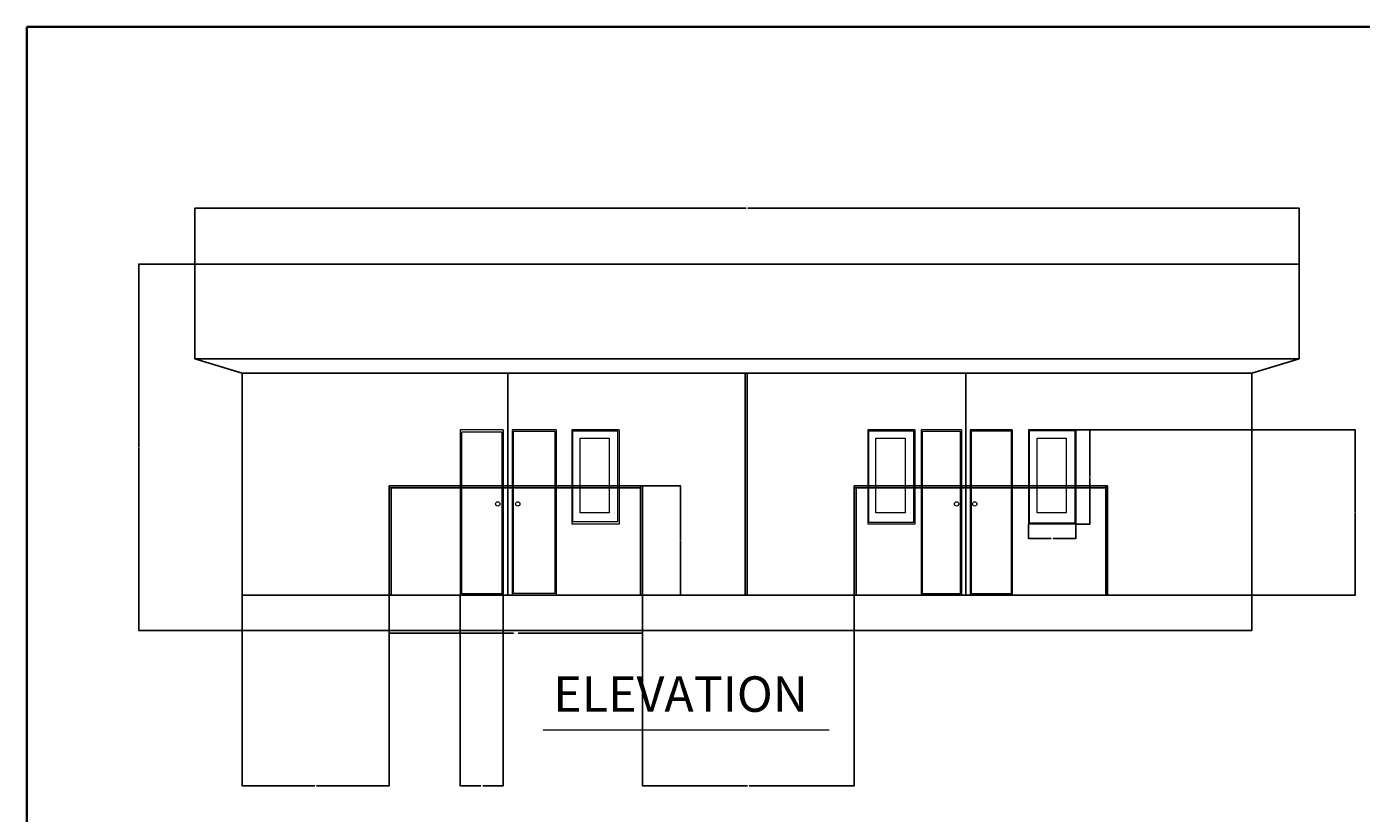
# Model space of a CAD drawing. Units: inches. Extents: x 2055 to 3558, y 1520 to 2888.
# Tile 4 of 8: x 2055 to 2732, y 2489 to 2888. Entities that reach past the tile are written whole.
import ezdxf

# ---------------------------------------------------------------- set-up
doc = ezdxf.new("R2010")
doc.units = ezdxf.units.IN
for name, color, linetype, lineweight in [('A-ANNO-DIMS', 2, 'Continuous', 18), ('A-ANNO-TEXT', 7, 'Continuous', 18), ('A-ANNO-TTLB', 7, 'Continuous', 35), ('A-ELEV', 7, 'Continuous', 25), ('A-ELEV-DOOR', 3, 'Continuous', 18), ('A-ELEV-GLAZ', 4, 'Continuous', 18)]:
    doc.layers.add(name, color=color, linetype=linetype, lineweight=lineweight)
doc.styles.get("Standard").update_dxf_attribs({"font": 'arial.ttf'})
doc.dimstyles.get("Standard").update_dxf_attribs({"dimtxt": 0.18, "dimasz": 0.18, "dimexe": 0.18, "dimexo": 0.0625, "dimgap": 0.09, "dimtad": 0, "dimtih": 1, "dimtoh": 1, "dimdec": 4, "dimzin": 0, "dimdsep": 46, "dimtxsty": 'Standard', "dimcen": 0.09, "dimadec": 0, "dimazin": 0, "dimtfac": 1, "dimtdec": 4, "dimtofl": 0, "dimtmove": 0, "dimatfit": 3, "dimfxl": 1, "dimtolj": 1, "dimtzin": 0, "dimarcsym": 0})

# ---------------------------------------------------------------- blocks, each defined once
blk = doc.blocks.new('VERANDA-FRONT-ELEV')
for p, q in [((0, 0), (0, 55.52)), ((0, 55.52), (128.65, 55.52)), ((127.65, 54.52), (0, 54.52)), ((0, 54.52), (1, 54.52)), ((1, 54.52), (1, 0)), ((127.65, 0), (127.65, 55.52)), ((127.65, 55.52), (127.65, 54.52)), ((128.65, 0), (128.65, 55.52)), ((128.65, 0), (127.65, 0))]:
    blk.add_line(p, q)
blk = doc.blocks.new('WIN-FRAME-ELEV-24')
for p, q in [((0, 48), (0, 0)), ((24, 48), (0, 48)), ((24, 48), (24, 0)), ((24, 0), (0, 0))]:
    blk.add_line(p, q)
blk = doc.blocks.new('*D50')
at = {"layer": 'A-ANNO-DIMS', "color": 0, "lineweight": -2, "transparency": 16777216}
for p, q in [((2587.37, 2683.6), (2594.69, 2683.6)), ((2594.51, 2683.42), (2594.51, 2659.78)), ((2594.51, 2635.78), (2594.51, 2659.42)), ((2587.37, 2635.6), (2594.69, 2635.6))]:
    blk.add_line(p, q, dxfattribs=at)
at = {"layer": 'A-ANNO-DIMS', "color": 0, "transparency": 16777216}
for points in [[(2594.48, 2683.42), (2594.54, 2683.42), (2594.51, 2683.6)], [(2594.48, 2635.78), (2594.54, 2635.78), (2594.51, 2635.6)]]:
    blk.add_solid(points, dxfattribs=at)
at = {"layer": 'Defpoints', "color": 0, "transparency": 16777216}
for p in [(2587.31, 2683.6), (2594.51, 2683.6), (2587.31, 2635.6)]:
    blk.add_point(p, dxfattribs=at)
at = {"layer": 'A-ANNO-DIMS', "color": 0, "transparency": 16777216, "insert": (2594.51, 2659.6), "char_height": 0.18, "attachment_point": 5}
blk.add_mtext('\\A1;WINDOW 48 TYP.', dxfattribs=at)
blk = doc.blocks.new('*D51')
at = {"layer": 'A-ANNO-DIMS', "color": 0, "lineweight": -2, "transparency": 16777216}
for p, q in [((2563.31, 2635.54), (2563.31, 2628.22)), ((2587.31, 2635.54), (2587.31, 2628.22)), ((2563.49, 2628.4), (2574.78, 2628.4)), ((2587.13, 2628.4), (2575.84, 2628.4))]:
    blk.add_line(p, q, dxfattribs=at)
at = {"layer": 'A-ANNO-DIMS', "color": 0, "transparency": 16777216}
for points in [[(2563.49, 2628.43), (2563.49, 2628.37), (2563.31, 2628.4)], [(2587.13, 2628.43), (2587.13, 2628.37), (2587.31, 2628.4)]]:
    blk.add_solid(points, dxfattribs=at)
at = {"layer": 'Defpoints', "color": 0, "transparency": 16777216}
for p in [(2563.31, 2635.6), (2587.31, 2635.6), (2587.31, 2628.4)]:
    blk.add_point(p, dxfattribs=at)
at = {"layer": 'A-ANNO-DIMS', "color": 0, "transparency": 16777216, "insert": (2575.31, 2628.4), "char_height": 0.18, "attachment_point": 5}
blk.add_mtext('\\A1;24 TYP.', dxfattribs=at)
blk = doc.blocks.new('*D116')
at = {"layer": 'A-ANNO-DIMS', "color": 0, "lineweight": -2, "transparency": 16777216}
for p, q in [((2238.74, 2599.54), (2238.74, 2580.12)), ((2367.39, 2599.54), (2367.39, 2580.12)), ((2238.92, 2580.3), (2301.82, 2580.3)), ((2367.21, 2580.3), (2304.31, 2580.3))]:
    blk.add_line(p, q, dxfattribs=at)
at = {"layer": 'A-ANNO-DIMS', "color": 0, "transparency": 16777216}
for points in [[(2238.92, 2580.33), (2238.92, 2580.27), (2238.74, 2580.3)], [(2367.21, 2580.33), (2367.21, 2580.27), (2367.39, 2580.3)]]:
    blk.add_solid(points, dxfattribs=at)
at = {"layer": 'Defpoints', "color": 0, "transparency": 16777216}
for p in [(2238.74, 2599.6), (2367.39, 2599.6), (2367.39, 2580.3)]:
    blk.add_point(p, dxfattribs=at)
at = {"layer": 'A-ANNO-DIMS', "color": 0, "transparency": 16777216, "insert": (2303.07, 2580.3), "char_height": 0.18, "attachment_point": 5}
blk.add_mtext('\\A1;VERANDA 129 TYP.', dxfattribs=at)
blk = doc.blocks.new('*D117')
at = {"layer": 'A-ANNO-DIMS', "color": 0, "lineweight": -2, "transparency": 16777216}
for p, q in [((2367.45, 2655.12), (2386.87, 2655.12)), ((2386.69, 2654.94), (2386.69, 2627.54)), ((2386.69, 2599.78), (2386.69, 2627.18)), ((2367.45, 2599.6), (2386.87, 2599.6))]:
    blk.add_line(p, q, dxfattribs=at)
at = {"layer": 'A-ANNO-DIMS', "color": 0, "transparency": 16777216}
for points in [[(2386.66, 2654.94), (2386.72, 2654.94), (2386.69, 2655.12)], [(2386.66, 2599.78), (2386.72, 2599.78), (2386.69, 2599.6)]]:
    blk.add_solid(points, dxfattribs=at)
at = {"layer": 'Defpoints', "color": 0, "transparency": 16777216}
for p in [(2367.39, 2655.12), (2386.69, 2655.12), (2367.39, 2599.6)]:
    blk.add_point(p, dxfattribs=at)
at = {"layer": 'A-ANNO-DIMS', "color": 0, "transparency": 16777216, "insert": (2386.69, 2627.36), "char_height": 0.18, "attachment_point": 5}
blk.add_mtext('\\A1;56 TYP.', dxfattribs=at)
blk = doc.blocks.new('*D143')
at = {"layer": 'A-ANNO-DIMS', "color": 0, "lineweight": -2, "transparency": 16777216}
for p, q in [((2140.17, 2767.66), (2140.17, 2796.23)), ((2140.35, 2796.05), (2420.03, 2796.05)), ((2700.49, 2796.05), (2420.82, 2796.05)), ((2700.67, 2767.66), (2700.67, 2796.23))]:
    blk.add_line(p, q, dxfattribs=at)
at = {"layer": 'A-ANNO-DIMS', "color": 0, "transparency": 16777216}
for points in [[(2140.35, 2796.08), (2140.35, 2796.02), (2140.17, 2796.05)], [(2700.49, 2796.08), (2700.49, 2796.02), (2700.67, 2796.05)]]:
    blk.add_solid(points, dxfattribs=at)
at = {"layer": 'Defpoints', "color": 0, "transparency": 16777216}
for p in [(2700.67, 2796.05), (2140.17, 2767.6), (2700.67, 2767.6)]:
    blk.add_point(p, dxfattribs=at)
at = {"layer": 'A-ANNO-DIMS', "color": 0, "transparency": 16777216, "insert": (2420.42, 2796.05), "char_height": 0.18, "attachment_point": 5}
blk.add_mtext('\\A1;560.5', dxfattribs=at)
blk = doc.blocks.new('*D144')
at = {"layer": 'A-ANNO-DIMS', "color": 0, "lineweight": -2, "transparency": 16777216}
for p, q in [((2140.11, 2767.6), (2111.54, 2767.6)), ((2111.72, 2767.42), (2111.72, 2674.78)), ((2111.72, 2581.78), (2111.72, 2674.42)), ((2164.11, 2581.6), (2111.54, 2581.6))]:
    blk.add_line(p, q, dxfattribs=at)
at = {"layer": 'A-ANNO-DIMS', "color": 0, "transparency": 16777216}
for points in [[(2111.69, 2767.42), (2111.75, 2767.42), (2111.72, 2767.6)], [(2111.69, 2581.78), (2111.75, 2581.78), (2111.72, 2581.6)]]:
    blk.add_solid(points, dxfattribs=at)
at = {"layer": 'Defpoints', "color": 0, "transparency": 16777216}
for p in [(2111.72, 2767.6), (2140.17, 2767.6), (2164.17, 2581.6)]:
    blk.add_point(p, dxfattribs=at)
at = {"layer": 'A-ANNO-DIMS', "color": 0, "transparency": 16777216, "insert": (2111.72, 2674.6), "char_height": 0.18, "attachment_point": 5}
blk.add_mtext('\\A1;186', dxfattribs=at)
blk = doc.blocks.new('*D145')
at = {"layer": 'A-ANNO-DIMS', "color": 0, "lineweight": -2, "transparency": 16777216}
for p, q in [((2164.17, 2599.54), (2164.17, 2502.58)), ((2238.74, 2599.54), (2238.74, 2502.58)), ((2164.35, 2502.76), (2201.07, 2502.76)), ((2238.56, 2502.76), (2201.85, 2502.76))]:
    blk.add_line(p, q, dxfattribs=at)
at = {"layer": 'A-ANNO-DIMS', "color": 0, "transparency": 16777216}
for points in [[(2164.35, 2502.79), (2164.35, 2502.73), (2164.17, 2502.76)], [(2238.56, 2502.79), (2238.56, 2502.73), (2238.74, 2502.76)]]:
    blk.add_solid(points, dxfattribs=at)
at = {"layer": 'Defpoints', "color": 0, "transparency": 16777216}
for p in [(2164.17, 2599.6), (2238.74, 2599.6), (2238.74, 2502.76)]:
    blk.add_point(p, dxfattribs=at)
at = {"layer": 'A-ANNO-DIMS', "color": 0, "transparency": 16777216, "insert": (2201.46, 2502.76), "char_height": 0.18, "attachment_point": 5}
blk.add_mtext('\\A1;74.57', dxfattribs=at)
blk = doc.blocks.new('*D146')
at = {"layer": 'A-ANNO-DIMS', "color": 0, "lineweight": -2, "transparency": 16777216}
for p, q in [((2367.39, 2599.54), (2367.39, 2502.58)), ((2474.84, 2599.54), (2474.84, 2502.58)), ((2367.57, 2502.76), (2420.66, 2502.76)), ((2474.66, 2502.76), (2421.57, 2502.76))]:
    blk.add_line(p, q, dxfattribs=at)
at = {"layer": 'A-ANNO-DIMS', "color": 0, "transparency": 16777216}
for points in [[(2367.57, 2502.79), (2367.57, 2502.73), (2367.39, 2502.76)], [(2474.66, 2502.79), (2474.66, 2502.73), (2474.84, 2502.76)]]:
    blk.add_solid(points, dxfattribs=at)
at = {"layer": 'Defpoints', "color": 0, "transparency": 16777216}
for p in [(2367.39, 2599.6), (2474.84, 2599.6), (2474.84, 2502.76)]:
    blk.add_point(p, dxfattribs=at)
at = {"layer": 'A-ANNO-DIMS', "color": 0, "transparency": 16777216, "insert": (2421.12, 2502.76), "char_height": 0.18, "attachment_point": 5}
blk.add_mtext('\\A1;107.45', dxfattribs=at)
blk = doc.blocks.new('*D147')
at = {"layer": 'A-ANNO-DIMS', "color": 0, "lineweight": -2, "transparency": 16777216}
for p, q in [((2274.85, 2599.54), (2274.85, 2502.58)), ((2296.67, 2599.54), (2296.67, 2502.58)), ((2275.03, 2502.76), (2285.3, 2502.76)), ((2296.49, 2502.76), (2286.23, 2502.76))]:
    blk.add_line(p, q, dxfattribs=at)
at = {"layer": 'A-ANNO-DIMS', "color": 0, "transparency": 16777216}
for points in [[(2275.03, 2502.79), (2275.03, 2502.73), (2274.85, 2502.76)], [(2296.49, 2502.79), (2296.49, 2502.73), (2296.67, 2502.76)]]:
    blk.add_solid(points, dxfattribs=at)
at = {"layer": 'Defpoints', "color": 0, "transparency": 16777216}
for p in [(2274.85, 2599.6), (2296.67, 2599.6), (2296.67, 2502.76)]:
    blk.add_point(p, dxfattribs=at)
at = {"layer": 'A-ANNO-DIMS', "color": 0, "transparency": 16777216, "insert": (2285.76, 2502.76), "char_height": 0.18, "attachment_point": 5}
blk.add_mtext('\\A1;21.824', dxfattribs=at)
blk = doc.blocks.new('*D148')
at = {"layer": 'A-ANNO-DIMS', "color": 0, "lineweight": -2, "transparency": 16777216}
for p, q in [((2587.37, 2683.6), (2729.3, 2683.6)), ((2729.12, 2683.42), (2729.12, 2641.78)), ((2729.12, 2599.78), (2729.12, 2641.42)), ((2603.55, 2599.6), (2729.3, 2599.6))]:
    blk.add_line(p, q, dxfattribs=at)
at = {"layer": 'A-ANNO-DIMS', "color": 0, "transparency": 16777216}
for points in [[(2729.09, 2683.42), (2729.15, 2683.42), (2729.12, 2683.6)], [(2729.09, 2599.78), (2729.15, 2599.78), (2729.12, 2599.6)]]:
    blk.add_solid(points, dxfattribs=at)
at = {"layer": 'Defpoints', "color": 0, "transparency": 16777216}
for p in [(2587.31, 2683.6), (2603.49, 2599.6), (2729.12, 2599.6)]:
    blk.add_point(p, dxfattribs=at)
at = {"layer": 'A-ANNO-DIMS', "color": 0, "transparency": 16777216, "insert": (2729.12, 2641.6), "char_height": 0.18, "attachment_point": 5}
blk.add_mtext('\\A1;84', dxfattribs=at)

msp = doc.modelspace()

# ---------------------------------------------------------------- linework, layer by layer
at = {"layer": 'A-ANNO-TEXT'}
msp.add_line((2316.9856, 2531.2058), (2462.068, 2531.2058), dxfattribs=at)
at = {"layer": 'A-ANNO-TTLB'}
msp.add_lwpolyline([(2054.7598, 2888.2545), (3557.8479, 2888.2545), (3557.8479, 1520.3256), (2054.7598, 1520.3256)], close=True, dxfattribs=at)
at = {"layer": 'A-ELEV'}
for p, q in [((2140.1747, 2719.5987), (2140.1747, 2767.5987)), ((2140.1747, 2767.5987), (2164.1747, 2767.5987)), ((2676.6747, 2767.5987), (2164.1747, 2767.5987)), ((2700.6747, 2767.5987), (2676.6747, 2767.5987)), ((2700.6747, 2719.5987), (2700.6747, 2767.5987)), ((2164.1747, 2719.5987), (2140.1747, 2719.5987)), ((2164.1747, 2712.2671), (2140.1747, 2719.5987)), ((2676.6747, 2719.5987), (2164.1747, 2719.5987)), ((2676.6747, 2719.5987), (2700.6747, 2719.5987)), ((2676.6747, 2712.2671), (2700.6747, 2719.5987)), ((2164.1747, 2712.2671), (2164.1747, 2581.5987)), ((2164.1747, 2712.2671), (2676.6747, 2712.2671)), ((2298.9868, 2599.5987), (2298.9868, 2712.2671)), ((2419.4247, 2599.5987), (2419.4247, 2712.2671)), ((2420.4247, 2599.5987), (2420.4247, 2712.2671)), ((2531.4812, 2599.5987), (2531.4812, 2712.2671)), ((2676.6747, 2712.2671), (2676.6747, 2581.5987)), ((2676.6747, 2599.5987), (2164.1747, 2599.5987)), ((2420.4247, 2599.5987), (2419.4247, 2599.5987)), ((2676.6747, 2581.5987), (2164.1747, 2581.5987))]:
    msp.add_line(p, q, dxfattribs=at)
at = {"layer": 'A-ELEV-DOOR'}
for p, q in [((2274.8511, 2683.5987), (2274.8511, 2599.5987)), ((2296.6747, 2683.5987), (2274.8511, 2683.5987)), ((2296.6747, 2683.5987), (2296.6747, 2599.5987)), ((2301.1747, 2683.5987), (2301.1747, 2599.5987)), ((2323.5061, 2683.5987), (2301.1747, 2683.5987)), ((2323.5061, 2683.5987), (2323.5061, 2599.5987)), ((2508.8547, 2683.5987), (2508.8547, 2599.5987)), ((2529.2739, 2683.5987), (2508.8547, 2683.5987)), ((2529.2739, 2683.5987), (2529.2739, 2599.5987)), ((2533.7739, 2683.5987), (2533.7739, 2599.5987)), ((2554.9501, 2683.5987), (2533.7739, 2683.5987)), ((2554.9501, 2683.5987), (2554.9501, 2599.5987))]:
    msp.add_line(p, q, dxfattribs=at)
for points in [[(2301.8083, 2682.9332), (2322.8572, 2682.9332), (2322.8572, 2600.3809), (2301.8083, 2600.3809)], [(2509.4418, 2682.8933), (2528.614, 2682.8933), (2528.614, 2600.1915), (2509.4418, 2600.1915)], [(2534.4144, 2683.0413), (2554.5708, 2683.0413), (2554.5708, 2600.3285), (2534.4144, 2600.3285)], [(2275.6674, 2682.6011), (2295.882, 2682.6011), (2295.882, 2600.2382), (2275.6674, 2600.2382)]]:
    msp.add_lwpolyline(points, close=True, dxfattribs=at)
for centre in [(2293.8771, 2645.9216), (2304.064, 2645.9216), (2526.7921, 2645.9216), (2536.044, 2645.9216)]:
    msp.add_circle(centre, 1.109, dxfattribs=at)
at = {"layer": 'A-ELEV-GLAZ'}
for points in [[(2332.018, 2683.0148), (2354.6702, 2683.0148), (2354.6702, 2636.7803), (2332.018, 2636.7803)], [(2482.2597, 2683.0015), (2505.0023, 2683.0015), (2505.0023, 2636.5724), (2482.2597, 2636.5724)], [(2563.7478, 2683.1536), (2586.785, 2683.1536), (2586.785, 2636.2117), (2563.7478, 2636.2117)], [(2335.7135, 2679.2744), (2350.4676, 2679.2744), (2350.4676, 2641.3596), (2335.7135, 2641.3596)], [(2485.8778, 2679.2744), (2500.632, 2679.2744), (2500.632, 2641.3596), (2485.8778, 2641.3596)], [(2567.7539, 2679.2744), (2582.508, 2679.2744), (2582.508, 2641.3596), (2567.7539, 2641.3596)]]:
    msp.add_lwpolyline(points, close=True, dxfattribs=at)

# ---------------------------------------------------------------- block references
at = {"layer": 'A-ELEV'}
for p in [(2238.745, 2599.599), (2474.8449, 2599.599)]:
    msp.add_blockref('VERANDA-FRONT-ELEV', p, dxfattribs=at)
at = {"layer": 'A-ELEV-GLAZ'}
for p in [(2331.54, 2635.599), (2481.6859, 2635.599), (2563.3126, 2635.599)]:
    msp.add_blockref('WIN-FRAME-ELEV-24', p, dxfattribs=at)

# ---------------------------------------------------------------- texts
at = {"layer": 'A-ANNO-TEXT', "insert": (2322.0614, 2558.3687), "char_height": 18, "attachment_point": 1}
msp.add_mtext_dynamic_manual_height_columns('ELEVATION', width=271.091415, gutter_width=12.5, heights=[0], dxfattribs=at)

# ---------------------------------------------------------------- dimensions: what is measured, and where the dimension line sits
at = {"layer": 'A-ANNO-DIMS'}
for base, p1, p2, override, picture, middle in [((2700.6747, 2796.0487), (2140.1747, 2767.5987), (2700.6747, 2767.5987), {"dimdec": 1, "dimlfac": 1, "dimrnd": 0, "dimzin": 0, "dimdsep": 46, "dimlunit": 2}, '*D143', (2420.4247, 2796.0487)), ((2238.745, 2502.7558), (2164.1747, 2599.5987), (2238.745, 2599.5987), {"dimdec": 2, "dimlfac": 1, "dimrnd": 0, "dimzin": 0, "dimdsep": 46, "dimlunit": 2}, '*D145', (2201.4598, 2502.7558)), ((2296.6747, 2502.7558), (2274.8511, 2599.5987), (2296.6747, 2599.5987), {"dimdec": 3, "dimlfac": 1, "dimrnd": 0, "dimzin": 0, "dimdsep": 46, "dimlunit": 2}, '*D147', (2285.7629, 2502.7558)), ((2474.8449, 2502.7558), (2367.3911, 2599.5987), (2474.8449, 2599.5987), {"dimdec": 2, "dimlfac": 1, "dimrnd": 0, "dimzin": 0, "dimdsep": 46, "dimlunit": 2}, '*D146', (2421.118, 2502.7558))]:
    dim = msp.add_linear_dim(base=base, p1=p1, p2=p2, dimstyle='Standard', override=override, dxfattribs=at)
    dim.commit()
    dim.dimension.update_dxf_attribs({"geometry": picture, "text_midpoint": middle})
for base, p1, p2, picture, middle in [((2111.7247, 2767.5987), (2164.1747, 2581.5987), (2140.1747, 2767.5987), '*D144', (2111.7247, 2674.5987)), ((2729.1247, 2599.5987), (2587.3124, 2683.5987), (2603.491, 2599.5987), '*D148', (2729.1247, 2641.5987))]:
    dim = msp.add_linear_dim(base=base, p1=p1, p2=p2, angle=90, dimstyle='Standard', override={"dimdec": 0, "dimlfac": 1, "dimrnd": 0, "dimzin": 0, "dimdsep": 46, "dimlunit": 2}, dxfattribs=at)
    dim.commit()
    dim.dimension.update_dxf_attribs({"geometry": picture, "text_midpoint": middle})
for base, p1, p2, text, picture, middle in [((2594.5124, 2683.5987), (2587.3124, 2635.5987), (2587.3124, 2683.5987), 'WINDOW <> TYP.', '*D50', (2594.5124, 2659.5987)), ((2386.6881, 2655.1228), (2367.3911, 2599.5987), (2367.3911, 2655.1228), '<> TYP.', '*D117', (2386.6881, 2627.3607))]:
    dim = msp.add_linear_dim(base=base, p1=p1, p2=p2, angle=90, text=text, dimstyle='Standard', override={"dimdec": 0, "dimlfac": 1, "dimrnd": 0, "dimzin": 0, "dimdsep": 46, "dimlunit": 2}, dxfattribs=at)
    dim.commit()
    dim.dimension.update_dxf_attribs({"geometry": picture, "text_midpoint": middle})
for base, p1, p2, text, picture, middle in [((2587.3124, 2628.3987), (2563.3124, 2635.5987), (2587.3124, 2635.5987), '<> TYP.', '*D51', (2575.3124, 2628.3987)), ((2367.3911, 2580.3018), (2238.745, 2599.5987), (2367.3911, 2599.5987), 'VERANDA <> TYP.', '*D116', (2303.0681, 2580.3018))]:
    dim = msp.add_linear_dim(base=base, p1=p1, p2=p2, text=text, dimstyle='Standard', override={"dimdec": 0, "dimlfac": 1, "dimrnd": 0, "dimzin": 0, "dimdsep": 46, "dimlunit": 2}, dxfattribs=at)
    dim.commit()
    dim.dimension.update_dxf_attribs({"geometry": picture, "text_midpoint": middle})

doc.saveas('drawing.dxf')
